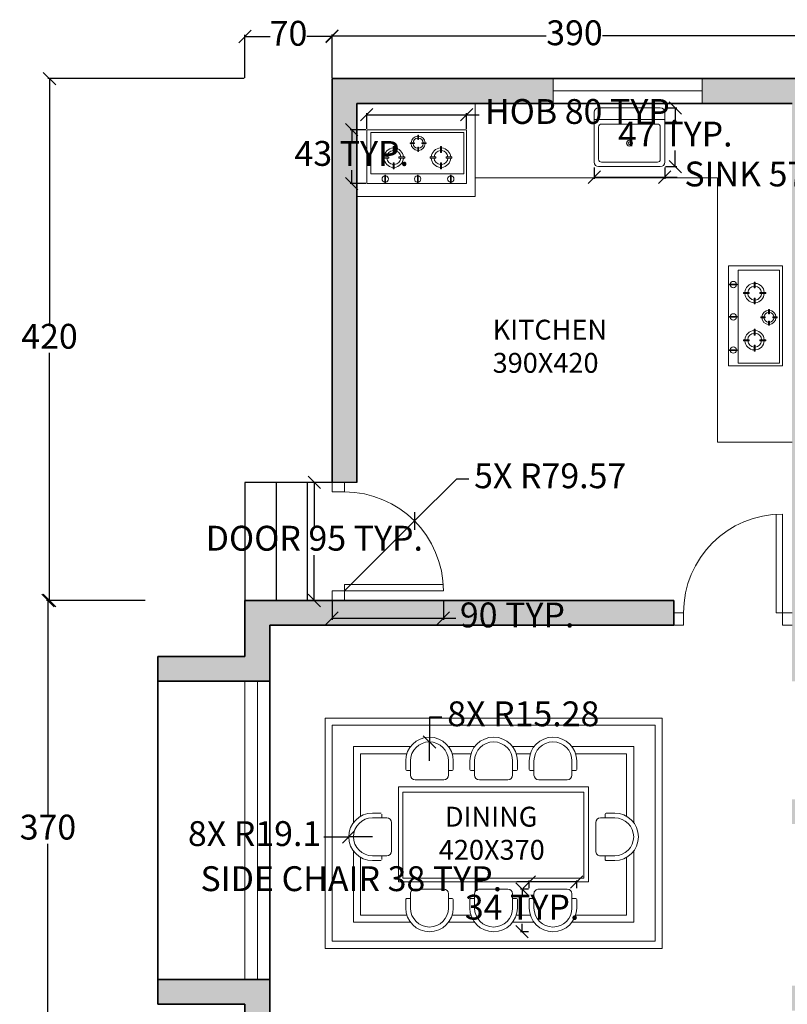
# Model space of a CAD drawing. Units: centimetres. Extents: x 2069 to 3209, y 376 to 1989.
# Tile 2 of 3: x 2069 to 2687, y 1196 to 1989. Entities that reach past the tile are written whole.
import ezdxf

# ---------------------------------------------------------------- set-up
doc = ezdxf.new("R2010")
doc.units = ezdxf.units.CM
for name, color, linetype, lineweight in [('A-ANNO-DIMS', 2, 'Continuous', 18), ('A-AREA-IDEN', 7, 'Continuous', 25), ('A-DOOR', 3, 'Continuous', 18), ('A-EQPM', 8, 'Continuous', 18), ('A-FLOR-CASE', 8, 'Continuous', 18), ('A-FLOR-FIXT', 8, 'Continuous', 18), ('A-FLOR-STRS', 7, 'Continuous', 25), ('A-FURN', 8, 'Continuous', 18), ('A-GLAZ', 4, 'Continuous', 18), ('A-WALL', 7, 'Continuous', 35), ('A-WALL-PATT', 252, 'Continuous', 13)]:
    doc.layers.add(name, color=color, linetype=linetype, lineweight=lineweight)
doc.styles.add('ATTR', font='romans.shx', dxfattribs={"width": 0.8, "height": 1.075})
doc.styles.get("Standard").update_dxf_attribs({"font": 'arial.ttf'})
doc.dimstyles.new('ISO-25', dxfattribs={"dimtxt": 20, "dimasz": 10, "dimexe": 1.25, "dimexo": 0.625, "dimtad": 0, "dimtih": 1, "dimtoh": 1, "dimtxsty": 'Standard', "dimblk": 'OBLIQUE', "dimcen": 6, "dimadec": 0, "dimazin": 0, "dimtfac": 1, "dimtmove": 0, "dimatfit": 3, "dimldrblk": 'OBLIQUE', "dimfxl": 1, "dimarcsym": 0})

# ---------------------------------------------------------------- blocks, each defined once
blk = doc.blocks.new("24'' Sink Single PV")
blk.add_line((-12.00001, -3.999996), (12, -3.999996))
for points in [[(-10.5, 0), (10.5, 0)], [(-12.00001, -18.499996), (-12.00001, -1.5)], [(12, -1.5), (12, -18.499996)], [(-10.5, -17.499996), (-10.5, -6.499996)], [(-9.5, -5.499996), (9.5, -5.499996)], [(10.5, -6.499996), (10.5, -17.499996)], [(10.5, -19.999996), (-10.5, -19.999996)], [(9.5, -18.499996), (-9.5, -18.499996)]]:
    blk.add_lwpolyline(points)
for radius in [1, 0.5]:
    blk.add_circle((0, -11.999996), radius)
for centre, radius, start, end in [((-10.5, -1.5), 1.5, 90, 180), ((10.5, -1.5), 1.5, 0, 90), ((-9.5, -6.499996), 1, 90, 180), ((9.5, -6.499996), 1, 0, 90), ((-10.5, -18.499996), 1.5, 180, 270), ((-9.5, -17.499996), 1, 180, 270), ((9.5, -17.499996), 1, 270, 0), ((10.5, -18.499996), 1.5, 270, 0)]:
    blk.add_arc(centre, radius, start, end)
at = {"style": 'ATTR', "width": 0.8, "flags": 9}
blk.add_attdef('ESTCODE', (0, 0), '', height=0.0048, dxfattribs=at)
blk = doc.blocks.new('A$C72243D80')
at = {"ltscale": 1000}
for p, q in [((0, 0), (0, 384.2)), ((0, 384.2), (712, 384.2)), ((29.5, 68.9), (29.5, 363.2)), ((29.5, 363.2), (692.7, 363.2)), ((692.7, 363.2), (692.7, 68.9)), ((712, 384.2), (712, 0)), ((309.4, 291), (340, 291)), ((309.4, 285), (309.4, 291)), ((340, 285), (309.4, 285)), ((340, 291), (340, 285)), ((363.5, 314.5), (363.5, 345.1)), ((363.5, 345.1), (369.5, 345.1)), ((369.5, 314.5), (363.5, 314.5)), ((369.5, 345.1), (369.5, 314.5)), ((392.3, 291), (392.3, 285)), ((422.9, 291), (392.3, 291)), ((392.3, 285), (422.9, 285)), ((422.9, 285), (422.9, 291)), ((188.1, 264.2), (188.1, 222.1)), ((196.4, 264.2), (188.1, 264.2)), ((188.1, 222.1), (196.4, 222.1)), ((196.4, 222.1), (196.4, 264.2)), ((363.5, 260), (363.5, 229.4)), ((369.5, 260), (363.5, 260)), ((363.5, 229.4), (369.5, 229.4)), ((369.5, 229.4), (369.5, 260)), ((525.9, 222.1), (525.9, 264.2)), ((525.9, 264.2), (534.1, 264.2)), ((534.1, 222.1), (525.9, 222.1)), ((534.1, 264.2), (534.1, 222.1)), ((114.7, 189.8), (156.8, 189.8)), ((114.7, 181.6), (114.7, 189.8)), ((156.8, 181.6), (114.7, 181.6)), ((156.8, 189.8), (156.8, 181.6)), ((188.1, 147.2), (196.4, 147.2)), ((188.1, 105.1), (188.1, 147.2)), ((196.4, 147.2), (196.4, 105.1)), ((228.6, 189.8), (228.6, 181.6)), ((270.7, 189.8), (228.6, 189.8)), ((228.6, 181.6), (270.7, 181.6)), ((270.7, 181.6), (270.7, 189.8)), ((451.5, 189.8), (493.6, 189.8)), ((451.5, 181.6), (451.5, 189.8)), ((493.6, 181.6), (451.5, 181.6)), ((493.6, 189.8), (493.6, 181.6)), ((525.9, 147.2), (525.9, 105.1)), ((534.1, 147.2), (525.9, 147.2)), ((534.1, 105.1), (534.1, 147.2)), ((565.5, 189.8), (565.5, 181.6)), ((607.6, 189.8), (565.5, 189.8)), ((565.5, 181.6), (607.6, 181.6)), ((607.6, 181.6), (607.6, 189.8)), ((196.4, 105.1), (188.1, 105.1)), ((525.9, 105.1), (534.1, 105.1)), ((712, 0), (0, 0)), ((692.7, 68.9), (29.5, 68.9)), ((129.6, 61.1), (129.6, 5)), ((134.4, 61.1), (129.6, 61.1)), ((129.6, 5), (134.4, 5)), ((134.4, 5), (134.4, 61.1)), ((360.9, 5), (360.9, 61.1)), ((360.9, 61.1), (365.7, 61.1)), ((365.7, 5), (360.9, 5)), ((365.7, 61.1), (365.7, 5)), ((597, 5), (597, 61.1)), ((597, 61.1), (601.8, 61.1)), ((601.8, 5), (597, 5)), ((601.8, 61.1), (601.8, 5))]:
    blk.add_line(p, q, dxfattribs=at)
for centre, radius, start, end in [((366.2, 287.2), 50.3, 182.57829, 266.96555), ((366.2, 287.2), 50.3, 93.03445, 175.72709), ((366.1, 287.8), 36.3, 94.03738, 175.01421), ((366.1, 287.8), 36.3, 184.51534, 265.96262), ((366.2, 287.2), 50.3, 4.27291, 86.18384), ((366.1, 287.8), 36.3, 4.98579, 84.5356), ((366.1, 287.8), 36.3, 275.4644, 355.48466), ((366.2, 287.2), 50.3, 273.81616, 357.42171), ((192.7, 184.7), 69.2, 93.81616, 175.72709), ((192.9, 185.5), 49.9, 95.4644, 175.01421), ((192.7, 184.7), 69.2, 4.27291, 86.96555), ((192.9, 185.5), 49.9, 4.98579, 85.96262), ((529.5, 184.7), 69.2, 93.03445, 175.72709), ((529.4, 185.5), 49.9, 94.03738, 175.01421), ((529.5, 184.7), 69.2, 4.27291, 86.18384), ((529.4, 185.5), 49.9, 4.98579, 84.5356), ((192.7, 184.7), 69.2, 182.57829, 266.18384), ((192.9, 185.5), 49.9, 184.51534, 264.5356), ((192.9, 185.5), 49.9, 274.03738, 355.48466), ((192.7, 184.7), 69.2, 273.03445, 357.42171), ((529.5, 184.7), 69.2, 182.57829, 266.96555), ((529.4, 185.5), 49.9, 184.51534, 265.96262), ((529.5, 184.7), 69.2, 273.81616, 357.42171), ((529.4, 185.5), 49.9, 275.4644, 355.48466), ((132.3, 33.2), 22.5, 96.74526, 263.25474), ((132.3, 33.2), 22.5, 275.47893, 84.52107), ((363.1, 33.2), 22.5, 95.47893, 264.52107), ((363.1, 33.2), 22.5, 276.74526, 83.25474), ((599.2, 33.2), 22.5, 95.47893, 264.52107), ((599.2, 33.2), 22.5, 276.74526, 83.25474)]:
    blk.add_arc(centre, radius, start, end, dxfattribs=at)
blk = doc.blocks.new('_Oblique')
at = {"color": 0, "linetype": 'ByBlock', "lineweight": -2}
blk.add_line((-0.5, -0.5), (0.5, 0.5), dxfattribs=at)
blk = doc.blocks.new('*D11')
at = {"layer": 'A-ANNO-DIMS', "color": 0, "lineweight": -2, "transparency": 16777216}
for p, q in [((2320.39, 1941.81), (2320.39, 1976.68)), ((2320.39, 1975.43), (2492.71, 1975.43)), ((2710.39, 1975.43), (2538.06, 1975.43)), ((2710.39, 1941.81), (2710.39, 1976.68))]:
    blk.add_line(p, q, dxfattribs=at)
at = {"layer": 'Defpoints', "color": 0, "transparency": 16777216}
for p in [(2710.39, 1975.43), (2320.39, 1941.18), (2710.39, 1941.18)]:
    blk.add_point(p, dxfattribs=at)
at = {"layer": 'A-ANNO-DIMS', "color": 0, "lineweight": -2, "transparency": 16777216, "xscale": 10, "yscale": 10, "zscale": 10, "rotation": 180}
blk.add_blockref('_Oblique', (2320.39, 1975.43), dxfattribs=at)
at = {"layer": 'A-ANNO-DIMS', "color": 0, "lineweight": -2, "transparency": 16777216, "xscale": 10, "yscale": 10, "zscale": 10}
blk.add_blockref('_Oblique', (2710.39, 1975.43), dxfattribs=at)
at = {"layer": 'A-ANNO-DIMS', "color": 0, "transparency": 16777216, "insert": (2515.39, 1975.43), "char_height": 20, "attachment_point": 5}
blk.add_mtext('390', dxfattribs=at)
blk = doc.blocks.new('*D14')
at = {"layer": 'A-ANNO-DIMS', "color": 0, "lineweight": -2, "transparency": 16777216}
for p, q in [((2250.39, 1941.81), (2250.39, 1976.27)), ((2250.39, 1975.02), (2270.55, 1975.02)), ((2320.39, 1975.02), (2300.22, 1975.02)), ((2320.39, 1941.81), (2320.39, 1976.27))]:
    blk.add_line(p, q, dxfattribs=at)
at = {"layer": 'Defpoints', "color": 0, "transparency": 16777216}
for p in [(2320.39, 1975.02), (2250.39, 1941.18), (2320.39, 1941.18)]:
    blk.add_point(p, dxfattribs=at)
at = {"layer": 'A-ANNO-DIMS', "color": 0, "lineweight": -2, "transparency": 16777216, "xscale": 10, "yscale": 10, "zscale": 10, "rotation": 180}
blk.add_blockref('_Oblique', (2250.39, 1975.02), dxfattribs=at)
at = {"layer": 'A-ANNO-DIMS', "color": 0, "lineweight": -2, "transparency": 16777216, "xscale": 10, "yscale": 10, "zscale": 10}
blk.add_blockref('_Oblique', (2320.39, 1975.02), dxfattribs=at)
at = {"layer": 'A-ANNO-DIMS', "color": 0, "transparency": 16777216, "insert": (2285.39, 1975.02), "char_height": 20, "attachment_point": 5}
blk.add_mtext('70', dxfattribs=at)
blk = doc.blocks.new('*D20')
at = {"layer": 'A-ANNO-DIMS', "color": 0, "lineweight": -2, "transparency": 16777216}
for p, q in [((2249.76, 1941.18), (2091.91, 1941.18)), ((2093.16, 1941.18), (2093.16, 1742.02)), ((2093.16, 1521.18), (2093.16, 1720.35)), ((2170.21, 1521.18), (2091.91, 1521.18))]:
    blk.add_line(p, q, dxfattribs=at)
at = {"layer": 'Defpoints', "color": 0, "transparency": 16777216}
for p in [(2250.39, 1941.18), (2093.16, 1521.18), (2170.84, 1521.18)]:
    blk.add_point(p, dxfattribs=at)
at = {"layer": 'A-ANNO-DIMS', "color": 0, "lineweight": -2, "transparency": 16777216, "xscale": 10, "yscale": 10, "zscale": 10}
for p, rotation in [((2093.16, 1941.18), 90), ((2093.16, 1521.18), 270)]:
    blk.add_blockref('_Oblique', p, dxfattribs=dict(at, rotation=rotation))
at = {"layer": 'A-ANNO-DIMS', "color": 0, "transparency": 16777216, "insert": (2093.16, 1731.18), "char_height": 20, "attachment_point": 5}
blk.add_mtext('420', dxfattribs=at)
blk = doc.blocks.new('*D21')
at = {"layer": 'A-ANNO-DIMS', "color": 0, "lineweight": -2, "transparency": 16777216}
for p, q in [((2170.21, 1521.18), (2090.66, 1521.18)), ((2091.91, 1521.18), (2091.91, 1347.03)), ((2091.91, 1151.18), (2091.91, 1325.34)), ((2171.09, 1151.18), (2090.66, 1151.18))]:
    blk.add_line(p, q, dxfattribs=at)
at = {"layer": 'Defpoints', "color": 0, "transparency": 16777216}
for p in [(2170.84, 1521.18), (2091.91, 1151.18), (2171.71, 1151.18)]:
    blk.add_point(p, dxfattribs=at)
at = {"layer": 'A-ANNO-DIMS', "color": 0, "lineweight": -2, "transparency": 16777216, "xscale": 10, "yscale": 10, "zscale": 10}
for p, rotation in [((2091.91, 1521.18), 90), ((2091.91, 1151.18), 270)]:
    blk.add_blockref('_Oblique', p, dxfattribs=dict(at, rotation=rotation))
at = {"layer": 'A-ANNO-DIMS', "color": 0, "transparency": 16777216, "insert": (2091.91, 1336.18), "char_height": 20, "attachment_point": 5}
blk.add_mtext('370', dxfattribs=at)
blk = doc.blocks.new('CHAIR-DINING')
for p, q in [((0, 8.4), (0, 15.28)), ((3.82, 15.28), (3.82, 3.82)), ((34.38, 3.82), (34.38, 15.28)), ((38.2, 8.4), (38.2, 15.28)), ((0.76, 7.64), (3.82, 7.64)), ((34.38, 7.64), (37.43, 7.64)), ((7.64, 0), (30.56, 0))]:
    blk.add_line(p, q)
for centre, radius, start, end in [((19.1, 15.28), 19.1, 0, 180), ((19.1, 15.28), 15.28, 0.00007, 179.99993), ((0.76, 8.4), 0.764, 180, 270), ((37.43, 8.4), 0.764, 270, 0), ((7.64, 3.82), 3.82, 180, 270), ((30.56, 3.82), 3.82, 270, 0)]:
    blk.add_arc(centre, radius, start, end)
blk = doc.blocks.new('DOOR-SINGLE-950')
for p, q in [((82.28, 89.41), (82.28, 10)), ((87.28, 89.57), (87.28, 10)), ((0, 10), (7.71, 10)), ((7.71, 10), (7.71, 0)), ((82.28, 10), (87.28, 10)), ((95, 10), (87.28, 10)), ((87.28, 10), (87.28, 0)), ((7.71, 0), (0, 0)), ((87.28, 0), (95, 0))]:
    blk.add_line(p, q)
blk.add_arc((87.28, 10), 79.57, 90, 180)
blk = doc.blocks.new('*D28')
at = {"layer": 'A-ANNO-DIMS', "color": 0, "lineweight": -2, "transparency": 16777216}
for p, q in [((2478.99, 1294.68), (2468.99, 1294.68)), ((2478.99, 1289.57), (2478.99, 1295.93)), ((2517.18, 1294.68), (2478.99, 1294.68)), ((2517.18, 1289.57), (2517.18, 1295.93))]:
    blk.add_line(p, q, dxfattribs=at)
at = {"layer": 'Defpoints', "color": 0, "transparency": 16777216}
for p in [(2478.99, 1294.68), (2478.99, 1288.95), (2517.18, 1288.95)]:
    blk.add_point(p, dxfattribs=at)
at = {"layer": 'A-ANNO-DIMS', "color": 0, "lineweight": -2, "transparency": 16777216, "xscale": 10, "yscale": 10, "zscale": 10, "rotation": 180}
blk.add_blockref('_Oblique', (2478.99, 1294.68), dxfattribs=at)
at = {"layer": 'A-ANNO-DIMS', "color": 0, "lineweight": -2, "transparency": 16777216, "xscale": 10, "yscale": 10, "zscale": 10}
blk.add_blockref('_Oblique', (2517.18, 1294.68), dxfattribs=at)
at = {"layer": 'A-ANNO-DIMS', "color": 0, "transparency": 16777216, "insert": (2335.9, 1294.68), "char_height": 20, "attachment_point": 5}
blk.add_mtext('SIDE CHAIR 38 TYP.', dxfattribs=at)
blk = doc.blocks.new('*D29')
at = {"layer": 'A-ANNO-DIMS', "color": 0, "lineweight": -2, "transparency": 16777216}
for p, q in [((2478.36, 1288.95), (2472.01, 1288.95)), ((2473.26, 1288.95), (2473.26, 1282.6)), ((2473.26, 1254.57), (2473.26, 1260.91)), ((2478.36, 1254.57), (2472.01, 1254.57))]:
    blk.add_line(p, q, dxfattribs=at)
at = {"layer": 'Defpoints', "color": 0, "transparency": 16777216}
for p in [(2478.99, 1288.95), (2473.26, 1254.57), (2478.99, 1254.57)]:
    blk.add_point(p, dxfattribs=at)
at = {"layer": 'A-ANNO-DIMS', "color": 0, "lineweight": -2, "transparency": 16777216, "xscale": 10, "yscale": 10, "zscale": 10}
for p, rotation in [((2473.26, 1288.95), 90), ((2473.26, 1254.57), 270)]:
    blk.add_blockref('_Oblique', p, dxfattribs=dict(at, rotation=rotation))
at = {"layer": 'A-ANNO-DIMS', "color": 0, "transparency": 16777216, "insert": (2473.26, 1271.76), "char_height": 20, "attachment_point": 5}
blk.add_mtext('34 TYP.', dxfattribs=at)
blk = doc.blocks.new('*D30')
at = {"layer": 'A-ANNO-DIMS', "color": 0, "lineweight": -2, "transparency": 16777216}
for p, q in [((2319.76, 1616.18), (2304.89, 1616.18)), ((2306.14, 1616.18), (2306.14, 1579.65)), ((2306.14, 1521.18), (2306.14, 1557.71)), ((2319.76, 1521.18), (2304.89, 1521.18))]:
    blk.add_line(p, q, dxfattribs=at)
at = {"layer": 'Defpoints', "color": 0, "transparency": 16777216}
for p in [(2320.39, 1616.18), (2306.14, 1521.18), (2320.39, 1521.18)]:
    blk.add_point(p, dxfattribs=at)
at = {"layer": 'A-ANNO-DIMS', "color": 0, "lineweight": -2, "transparency": 16777216, "xscale": 10, "yscale": 10, "zscale": 10}
for p, rotation in [((2306.14, 1616.18), 90), ((2306.14, 1521.18), 270)]:
    blk.add_blockref('_Oblique', p, dxfattribs=dict(at, rotation=rotation))
at = {"layer": 'A-ANNO-DIMS', "color": 0, "transparency": 16777216, "insert": (2306.14, 1568.68), "char_height": 20, "attachment_point": 5}
blk.add_mtext('DOOR 95 TYP.', dxfattribs=at)
blk = doc.blocks.new('*D31')
at = {"layer": 'A-ANNO-DIMS', "color": 0, "lineweight": -2, "transparency": 16777216}
for p, q in [((2320.39, 1520.56), (2320.39, 1505.68)), ((2409.96, 1520.56), (2409.96, 1505.68)), ((2320.39, 1506.93), (2409.96, 1506.93)), ((2409.96, 1506.93), (2419.96, 1506.93))]:
    blk.add_line(p, q, dxfattribs=at)
at = {"layer": 'Defpoints', "color": 0, "transparency": 16777216}
for p in [(2320.39, 1521.18), (2409.96, 1521.18), (2409.96, 1506.93)]:
    blk.add_point(p, dxfattribs=at)
at = {"layer": 'A-ANNO-DIMS', "color": 0, "lineweight": -2, "transparency": 16777216, "xscale": 10, "yscale": 10, "zscale": 10, "rotation": 180}
blk.add_blockref('_Oblique', (2320.39, 1506.93), dxfattribs=at)
at = {"layer": 'A-ANNO-DIMS', "color": 0, "lineweight": -2, "transparency": 16777216, "xscale": 10, "yscale": 10, "zscale": 10}
blk.add_blockref('_Oblique', (2409.96, 1506.93), dxfattribs=at)
at = {"layer": 'A-ANNO-DIMS', "color": 0, "transparency": 16777216, "insert": (2469.26, 1506.93), "char_height": 20, "attachment_point": 5}
blk.add_mtext('90 TYP.', dxfattribs=at)
blk = doc.blocks.new('*D36')
at = {"layer": 'A-ANNO-DIMS', "color": 0, "lineweight": -2, "transparency": 16777216}
for p, q in [((2531.27, 1869.68), (2531.27, 1860.55)), ((2587.96, 1869.68), (2587.96, 1860.55)), ((2531.27, 1861.8), (2587.96, 1861.8)), ((2587.96, 1861.8), (2597.96, 1861.8))]:
    blk.add_line(p, q, dxfattribs=at)
at = {"layer": 'Defpoints', "color": 0, "transparency": 16777216}
for p in [(2531.27, 1870.31), (2587.96, 1870.31), (2587.96, 1861.8)]:
    blk.add_point(p, dxfattribs=at)
at = {"layer": 'A-ANNO-DIMS', "color": 0, "lineweight": -2, "transparency": 16777216, "xscale": 10, "yscale": 10, "zscale": 10, "rotation": 180}
blk.add_blockref('_Oblique', (2531.27, 1861.8), dxfattribs=at)
at = {"layer": 'A-ANNO-DIMS', "color": 0, "lineweight": -2, "transparency": 16777216, "xscale": 10, "yscale": 10, "zscale": 10}
blk.add_blockref('_Oblique', (2587.96, 1861.8), dxfattribs=at)
at = {"layer": 'A-ANNO-DIMS', "color": 0, "transparency": 16777216, "insert": (2683.7, 1861.8), "char_height": 20, "attachment_point": 5}
blk.add_mtext('SINK 57 TYP.', dxfattribs=at)
blk = doc.blocks.new('*D37')
at = {"layer": 'A-ANNO-DIMS', "color": 0, "lineweight": -2, "transparency": 16777216}
for p, q in [((2588.59, 1917.56), (2597.72, 1917.56)), ((2596.47, 1917.56), (2596.47, 1904.57)), ((2596.47, 1870.31), (2596.47, 1883.3)), ((2588.59, 1870.31), (2597.72, 1870.31))]:
    blk.add_line(p, q, dxfattribs=at)
at = {"layer": 'Defpoints', "color": 0, "transparency": 16777216}
for p in [(2587.96, 1917.56), (2596.47, 1917.56), (2587.96, 1870.31)]:
    blk.add_point(p, dxfattribs=at)
at = {"layer": 'A-ANNO-DIMS', "color": 0, "lineweight": -2, "transparency": 16777216, "xscale": 10, "yscale": 10, "zscale": 10}
for p, rotation in [((2596.47, 1917.56), 90), ((2596.47, 1870.31), 270)]:
    blk.add_blockref('_Oblique', p, dxfattribs=dict(at, rotation=rotation))
at = {"layer": 'A-ANNO-DIMS', "color": 0, "transparency": 16777216, "insert": (2596.47, 1893.93), "char_height": 20, "attachment_point": 5}
blk.add_mtext('47 TYP.', dxfattribs=at)
blk = doc.blocks.new('*D38')
at = {"layer": 'A-ANNO-DIMS', "color": 0, "lineweight": -2, "transparency": 16777216}
for p, q in [((2348.29, 1900.65), (2348.29, 1913.33)), ((2348.29, 1912.08), (2428.64, 1912.08)), ((2428.64, 1900.65), (2428.64, 1913.33)), ((2428.64, 1912.08), (2438.64, 1912.08))]:
    blk.add_line(p, q, dxfattribs=at)
at = {"layer": 'Defpoints', "color": 0, "transparency": 16777216}
for p in [(2428.64, 1912.08), (2348.29, 1900.03), (2428.64, 1900.03)]:
    blk.add_point(p, dxfattribs=at)
at = {"layer": 'A-ANNO-DIMS', "color": 0, "lineweight": -2, "transparency": 16777216, "xscale": 10, "yscale": 10, "zscale": 10, "rotation": 180}
blk.add_blockref('_Oblique', (2348.29, 1912.08), dxfattribs=at)
at = {"layer": 'A-ANNO-DIMS', "color": 0, "lineweight": -2, "transparency": 16777216, "xscale": 10, "yscale": 10, "zscale": 10}
blk.add_blockref('_Oblique', (2428.64, 1912.08), dxfattribs=at)
at = {"layer": 'A-ANNO-DIMS', "color": 0, "transparency": 16777216, "insert": (2521.55, 1912.08), "char_height": 20, "attachment_point": 5}
blk.add_mtext('HOB 80 TYP.', dxfattribs=at)
blk = doc.blocks.new('*D39')
at = {"layer": 'A-ANNO-DIMS', "color": 0, "lineweight": -2, "transparency": 16777216}
for p, q in [((2347.66, 1900.03), (2334.98, 1900.03)), ((2336.23, 1900.03), (2336.23, 1889.19)), ((2336.23, 1856.67), (2336.23, 1867.51)), ((2347.66, 1856.67), (2334.98, 1856.67))]:
    blk.add_line(p, q, dxfattribs=at)
at = {"layer": 'Defpoints', "color": 0, "transparency": 16777216}
for p in [(2336.23, 1900.03), (2348.29, 1900.03), (2348.29, 1856.67)]:
    blk.add_point(p, dxfattribs=at)
at = {"layer": 'A-ANNO-DIMS', "color": 0, "lineweight": -2, "transparency": 16777216, "xscale": 10, "yscale": 10, "zscale": 10}
for p, rotation in [((2336.23, 1900.03), 90), ((2336.23, 1856.67), 270)]:
    blk.add_blockref('_Oblique', p, dxfattribs=dict(at, rotation=rotation))
at = {"layer": 'A-ANNO-DIMS', "color": 0, "transparency": 16777216, "insert": (2336.23, 1878.35), "char_height": 20, "attachment_point": 5}
blk.add_mtext('43 TYP.', dxfattribs=at)
blk = doc.blocks.new('*D50')
at = {"layer": 'A-ANNO-DIMS', "color": 0, "lineweight": -2, "transparency": 16777216}
for p, q in [((2420.41, 1618.92), (2386.65, 1585.16)), ((2430.41, 1618.92), (2420.41, 1618.92)), ((2330.39, 1528.9), (2386.65, 1585.16))]:
    blk.add_line(p, q, dxfattribs=at)
at = {"layer": 'Defpoints', "color": 0, "transparency": 16777216}
for p in [(2386.65, 1585.16), (2330.39, 1528.9)]:
    blk.add_point(p, dxfattribs=at)
at = {"layer": 'A-ANNO-DIMS', "color": 0, "lineweight": -2, "transparency": 16777216, "xscale": 10, "yscale": 10, "zscale": 10, "rotation": 224.9997739305666}
blk.add_blockref('_Oblique', (2386.65, 1585.16), dxfattribs=at)
at = {"layer": 'A-ANNO-DIMS', "color": 0, "transparency": 16777216, "insert": (2495.84, 1618.92), "char_height": 20, "attachment_point": 5}
blk.add_mtext('5X R79.57', dxfattribs=at)
blk = doc.blocks.new('*D55')
at = {"layer": 'A-ANNO-DIMS', "color": 0, "lineweight": -2, "transparency": 16777216}
for p in [(2313.84, 1330.96), (2352.94, 1330.96)]:
    blk.add_line(p, (2333.84, 1330.96), dxfattribs=at)
at = {"layer": 'Defpoints', "color": 0, "transparency": 16777216}
for p in [(2333.84, 1330.96), (2352.94, 1330.96)]:
    blk.add_point(p, dxfattribs=at)
at = {"layer": 'A-ANNO-DIMS', "color": 0, "lineweight": -2, "transparency": 16777216, "xscale": 10, "yscale": 10, "zscale": 10, "rotation": 359.9994809913539}
blk.add_blockref('_Oblique', (2333.84, 1330.96), dxfattribs=at)
at = {"layer": 'A-ANNO-DIMS', "color": 0, "transparency": 16777216, "insert": (2258.1, 1330.96), "char_height": 20, "attachment_point": 5}
blk.add_mtext('8X R19.1', dxfattribs=at)
blk = doc.blocks.new('*D56')
at = {"layer": 'A-ANNO-DIMS', "color": 0, "lineweight": -2, "transparency": 16777216}
for p, q in [((2408.77, 1427.36), (2398.77, 1427.36)), ((2398.77, 1427.36), (2398.77, 1407.36)), ((2398.77, 1392.08), (2398.77, 1407.36))]:
    blk.add_line(p, q, dxfattribs=at)
at = {"layer": 'Defpoints', "color": 0, "transparency": 16777216}
for p in [(2398.77, 1407.36), (2398.77, 1392.08)]:
    blk.add_point(p, dxfattribs=at)
at = {"layer": 'A-ANNO-DIMS', "color": 0, "lineweight": -2, "transparency": 16777216, "xscale": 10, "yscale": 10, "zscale": 10, "rotation": 269.9993737395664}
blk.add_blockref('_Oblique', (2398.77, 1407.36), dxfattribs=at)
at = {"layer": 'A-ANNO-DIMS', "color": 0, "transparency": 16777216, "insert": (2474.23, 1427.36), "char_height": 20, "attachment_point": 5}
blk.add_mtext('8X R15.28', dxfattribs=at)

msp = doc.modelspace()

# ---------------------------------------------------------------- hatches: boundary and pattern name
at = {"layer": 'A-WALL-PATT'}
h = msp.add_hatch(color=256, dxfattribs=at)
h.dxf.hatch_style = 1
h.paths.add_polyline_path([(2498.1872, 1921.1819), (2498.1872, 1941.1819), (2320.3865, 1941.1819), (2320.3865, 1616.1819), (2340.3865, 1616.1819), (2340.3865, 1921.1819)])
h.paths.add_polyline_path([(2690.3865, 1921.1819), (2690.3865, 1456.1819), (2710.3865, 1456.1819), (2710.3865, 1741.1819), (2742.2674, 1741.1819), (2742.2674, 1761.1819), (2710.3865, 1761.1819), (2710.3865, 1941.1819), (2618.1872, 1941.1819), (2618.1872, 1921.1819)])
h.paths.add_polyline_path([(2802.2674, 1761.1819), (2802.2674, 1741.1819), (2971.3879, 1741.1819), (2971.3879, 1761.1819)])
h.paths.add_polyline_path([(3080.3865, 1761.1819), (3031.3879, 1761.1819), (3031.3879, 1741.1819), (3060.3865, 1741.1819), (3060.3865, 1621.1819), (3080.3865, 1621.1819)])
h.paths.add_polyline_path([(3060.3865, 1361.1819), (2906.9077, 1361.1819), (2906.9077, 1341.1819), (3060.3865, 1341.1819), (3060.3865, 1296.1819), (3080.3865, 1296.1819), (3080.3865, 1481.1819), (3060.3865, 1481.1819)])
h.paths.add_polyline_path([(2799.9077, 1341.1819), (2799.9077, 1211.1819), (2690.3865, 1211.1819), (2690.3865, 1191.1819), (3060.3865, 1191.1819), (3060.3865, 1131.1819), (3080.3865, 1131.1819), (3080.3865, 1256.1819), (3060.3865, 1256.1819), (3060.3865, 1211.1819), (2821.9077, 1211.1819), (2821.9077, 1361.1819), (2690.3865, 1361.1819), (2690.3865, 1341.1819)])
h.paths.add_polyline_path([(3080.3865, 1051.1819), (3060.3865, 1051.1819), (3060.3865, 991.1819), (2805.3865, 991.1819), (2805.3865, 971.1819), (3060.3865, 971.1819), (3060.3865, 861.1819), (3080.3865, 861.1819)])
h.paths.add_polyline_path([(2690.3865, 591.1819), (2815.3865, 591.1819), (2815.3865, 611.1819), (2710.3865, 611.1819), (2710.3865, 991.1819), (2690.3865, 991.1819)])
h.paths.add_polyline_path([(2955.3865, 611.1819), (2955.3865, 591.1819), (3080.3865, 591.1819), (3080.3865, 721.1819), (3060.3865, 721.1819), (3060.3865, 611.1819)])
h.paths.add_polyline_path([(2320.3865, 656.2562), (2320.3865, 639.1819), (2343.1963, 639.1819), (2343.1963, 656.2562)])
h.paths.add_polyline_path([(2320.3865, 863.2574), (2250.3865, 863.2574), (2250.3865, 841.2574), (2407.8865, 841.2574), (2407.8865, 863.2574), (2340.3865, 863.2574), (2340.3865, 927.2197), (2320.3865, 927.2197)])
h.paths.add_polyline_path([(2320.3865, 1151.1819), (2320.3865, 1087.2197), (2340.3865, 1087.2197), (2340.3865, 1151.1819), (2595.3865, 1151.1819), (2595.3865, 1171.1819), (2270.3865, 1171.1819), (2270.3865, 1216.1819), (2180.3865, 1216.1819), (2180.3865, 1196.1819), (2250.3865, 1196.1819), (2250.3865, 1151.1819)])
h.paths.add_polyline_path([(2595.3865, 1501.1819), (2595.3865, 1521.1819), (2250.3865, 1521.1819), (2250.3865, 1476.1819), (2180.3865, 1476.1819), (2180.3865, 1456.1819), (2270.3865, 1456.1819), (2270.3865, 1501.1819)])

# ---------------------------------------------------------------- linework, layer by layer
at = {"layer": 'A-FLOR-CASE'}
for p, q in [((2435.3865, 1921.1819), (2435.3865, 1846.1819)), ((2435.3865, 1861.1819), (2630.3865, 1861.1819)), ((2630.3865, 1861.1819), (2630.3865, 1648.6184)), ((2340.3865, 1846.1819), (2435.3865, 1846.1819)), ((2630.3865, 1648.6184), (2690.3865, 1648.6184))]:
    msp.add_line(p, q, dxfattribs=at)
at = {"layer": 'A-FLOR-STRS'}
for p, q in [((2340.3865, 1616.1819), (2250.3865, 1616.1819)), ((2250.3865, 1616.1819), (2250.3865, 1521.1819)), ((2275.3865, 1616.1819), (2275.3865, 1521.1819)), ((2300.3865, 1616.1819), (2300.3865, 1521.1819))]:
    msp.add_line(p, q, dxfattribs=at)
at = {"layer": 'A-FURN'}
for p, q in [((2585.9359, 1426.4542), (2314.7404, 1426.4542)), ((2314.7404, 1426.4542), (2314.7404, 1241.2009)), ((2585.9359, 1241.2009), (2585.9359, 1426.4542)), ((2580.2064, 1420.7247), (2320.4699, 1420.7247)), ((2320.4699, 1420.7247), (2320.4699, 1246.9304)), ((2580.2064, 1246.9304), (2580.2064, 1420.7247)), ((2383.4942, 1403.5363), (2337.6584, 1403.5363)), ((2337.6584, 1403.5363), (2337.6584, 1342.4218)), ((2435.0596, 1403.5363), (2414.0515, 1403.5363)), ((2482.8052, 1403.5363), (2465.6168, 1403.5363)), ((2563.018, 1403.5363), (2513.3625, 1403.5363)), ((2563.018, 1342.4218), (2563.018, 1403.5363)), ((2343.3878, 1397.8068), (2343.3878, 1347.5024)), ((2380.5542, 1397.8068), (2343.3878, 1397.8068)), ((2432.1196, 1397.8068), (2416.9914, 1397.8068)), ((2479.8653, 1397.8068), (2468.5568, 1397.8068)), ((2557.2885, 1397.8068), (2516.3025, 1397.8068)), ((2557.2885, 1347.5024), (2557.2885, 1397.8068)), ((2373.9451, 1294.6761), (2373.9451, 1371.0692)), ((2373.9451, 1371.0692), (2526.7313, 1371.0692)), ((2526.7313, 1371.0692), (2526.7313, 1294.6761)), ((2359.8124, 1350.0611), (2352.937, 1350.0611)), ((2360.5763, 1346.2414), (2360.5763, 1349.2972)), ((2364.3959, 1346.2414), (2352.937, 1346.2414)), ((2368.2156, 1319.5039), (2368.2156, 1342.4218)), ((2337.6584, 1319.5039), (2337.6584, 1262.209)), ((2352.937, 1315.6842), (2364.3959, 1315.6842)), ((2360.5763, 1312.6285), (2360.5763, 1315.6842)), ((2563.018, 1262.209), (2563.018, 1319.5039)), ((2343.3878, 1314.4232), (2343.3878, 1267.9385)), ((2359.8124, 1311.8646), (2352.937, 1311.8646)), ((2557.2885, 1267.9385), (2557.2885, 1314.4232)), ((2526.7313, 1294.6761), (2373.9451, 1294.6761)), ((2343.3878, 1267.9385), (2380.5542, 1267.9385)), ((2416.9914, 1267.9385), (2432.1196, 1267.9385)), ((2468.5568, 1267.9385), (2479.8653, 1267.9385)), ((2516.3025, 1267.9385), (2557.2885, 1267.9385)), ((2337.6584, 1262.209), (2383.4942, 1262.209)), ((2414.0515, 1262.209), (2435.0596, 1262.209)), ((2465.6168, 1262.209), (2482.8052, 1262.209)), ((2513.3625, 1262.209), (2563.018, 1262.209)), ((2320.4699, 1246.9304), (2580.2064, 1246.9304)), ((2314.7404, 1241.2009), (2585.9359, 1241.2009))]:
    msp.add_line(p, q, dxfattribs=at)
msp.add_lwpolyline([(2377.3409, 1366.9642), (2522.9512, 1366.9642), (2522.9512, 1297.7838), (2377.3409, 1297.7838)], close=True, dxfattribs=at)
for centre, radius, start, end in [((2352.937, 1330.9628), 19.0983, 90, 270), ((2352.937, 1330.9628), 15.2786, 90.0000737, 269.9999263), ((2364.3959, 1342.4218), 3.8197, 0, 90), ((2364.3959, 1319.5039), 3.8197, 270, 0)]:
    msp.add_arc(centre, radius, start, end, dxfattribs=at)
at = {"layer": 'A-GLAZ'}
for p, q in [((2498.1872, 1921.1819), (2498.1872, 1941.1819)), ((2618.1872, 1921.1819), (2618.1872, 1941.1819)), ((2498.1872, 1931.1819), (2618.1872, 1931.1819)), ((2250.3865, 1456.1819), (2250.3865, 1216.1819)), ((2260.3865, 1216.1819), (2260.3865, 1456.1819))]:
    msp.add_line(p, q, dxfattribs=at)
at = {"layer": 'A-WALL'}
for p, q in [((2320.3865, 1941.1819), (2710.3865, 1941.1819)), ((2320.3865, 1941.1819), (2320.3865, 1616.1819)), ((2340.3865, 1921.1819), (2690.3865, 1921.1819)), ((2340.3865, 1921.1819), (2340.3865, 1616.1819)), ((2595.3865, 1521.1819), (2250.3865, 1521.1819)), ((2250.3865, 1521.1819), (2250.3865, 1476.1819)), ((2595.3865, 1521.1819), (2595.3865, 1501.1819)), ((2595.3865, 1501.1819), (2270.3865, 1501.1819)), ((2270.3865, 1501.1819), (2270.3865, 1171.1819)), ((2180.3865, 1476.1819), (2180.3865, 1196.1819)), ((2250.3865, 1476.1819), (2180.3865, 1476.1819)), ((2270.3865, 1456.1819), (2180.3865, 1456.1819)), ((2270.3865, 1216.1819), (2180.3865, 1216.1819)), ((2250.3865, 1196.1819), (2180.3865, 1196.1819)), ((2250.3865, 1196.1819), (2250.3865, 841.2574))]:
    msp.add_line(p, q, dxfattribs=at)

# ---------------------------------------------------------------- block references
at = {"layer": 'A-DOOR', "rotation": 269.9999999999997}
msp.add_blockref('DOOR-SINGLE-950', (2320.3866, 1616.1815), dxfattribs=at)
at = {"layer": 'A-DOOR'}
msp.add_blockref('DOOR-SINGLE-950', (2595.387, 1501.182), dxfattribs=at)
at = {"layer": 'A-EQPM', "xscale": 0.1128460274394379, "yscale": 0.1128460274394379, "zscale": 0.1128460274394379}
msp.add_blockref('A$C72243D80', (2348.2865, 1856.6729), dxfattribs=at)
at = {"layer": 'A-EQPM', "xscale": 0.1128460274394379, "yscale": 0.1128460274394379, "zscale": 0.1128460274394379, "rotation": 270}
msp.add_blockref('A$C72243D80', (2639.3664, 1790.3423), dxfattribs=at)
at = {"layer": 'A-FLOR-FIXT', "xscale": 2.362111345995379, "yscale": 2.362111345995379, "zscale": 2.362111345995379}
msp.add_blockref("24'' Sink Single PV", (2559.6171, 1917.5491), dxfattribs=at)
at = {"layer": 'A-FURN'}
for p in [(2379.675, 1376.799), (2431.2403, 1376.799), (2478.986, 1376.799)]:
    msp.add_blockref('CHAIR-DINING', p, dxfattribs=at)
for p, rotation in [((2532.4611, 1350.0607), 270.000000000189), ((2417.8707, 1288.9463), 180), ((2469.436, 1288.9463), 180), ((2517.1817, 1288.9463), 180)]:
    msp.add_blockref('CHAIR-DINING', p, dxfattribs=dict(at, rotation=rotation))

# ---------------------------------------------------------------- texts
at = {"layer": 'A-AREA-IDEN', "char_height": 16, "attachment_point": 1}
for s, width, insert in [('KITCHEN\\P390X420', 109.524929, (2449.5532, 1747.0716)), (' DINING\\P420X370', 112.813406, (2406.2964, 1355.1715))]:
    msp.add_mtext_dynamic_manual_height_columns(s, width=width, gutter_width=12.5, heights=[0], dxfattribs=dict(at, insert=insert))

# ---------------------------------------------------------------- dimensions: what is measured, and where the dimension line sits
at = {"layer": 'A-ANNO-DIMS'}
for base, p1, p2, picture, middle in [((2320.3865, 1975.0194), (2250.3865, 1941.1819), (2320.3865, 1941.1819), '*D14', (2285.3865, 1975.0194)), ((2710.3865, 1975.4288), (2320.3865, 1941.1819), (2710.3865, 1941.1819), '*D11', (2515.3865, 1975.4288))]:
    dim = msp.add_linear_dim(base=base, p1=p1, p2=p2, dimstyle='ISO-25', override={"dimclrd": 0, "dimclre": 0, "dimclrt": 0}, dxfattribs=at)
    dim.commit()
    dim.dimension.update_dxf_attribs({"geometry": picture, "text_midpoint": middle})
for base, p1, p2, text, picture, middle in [((2428.638, 1912.0817), (2348.2865, 1900.029), (2428.638, 1900.029), 'HOB <> TYP.', '*D38', (2521.555, 1912.0817)), ((2587.9624, 1861.8033), (2531.2717, 1870.3069), (2587.9624, 1870.3069), 'SINK <> TYP.', '*D36', (2683.7034, 1861.8033)), ((2409.9564, 1506.9319), (2320.3865, 1521.1819), (2409.9564, 1521.1819), '<> TYP.', '*D31', (2469.2581, 1506.9319))]:
    dim = msp.add_linear_dim(base=base, p1=p1, p2=p2, text=text, dimstyle='ISO-25', override={"dimdec": 0, "dimlfac": 1, "dimrnd": 0, "dimzin": 0, "dimdsep": 46, "dimlunit": 2}, dxfattribs=at)
    dim.commit()
    dim.dimension.update_dxf_attribs({"geometry": picture, "text_midpoint": middle})
for base, p1, p2, picture, middle in [((2093.1605, 1521.1819), (2250.3865, 1941.1819), (2170.836, 1521.1819), '*D20', (2093.1605, 1731.1819)), ((2091.9105, 1151.1819), (2170.836, 1521.1819), (2171.711, 1151.1819), '*D21', (2091.9105, 1336.1819))]:
    dim = msp.add_linear_dim(base=base, p1=p1, p2=p2, angle=90, dimstyle='ISO-25', override={"dimclrd": 0, "dimclre": 0, "dimclrt": 0}, dxfattribs=at)
    dim.commit()
    dim.dimension.update_dxf_attribs({"geometry": picture, "text_midpoint": middle})
for base, p1, p2, angle, text, picture, middle in [((2596.466, 1917.5605), (2587.9624, 1870.3069), (2587.9624, 1917.5605), 90, '<> TYP.', '*D37', (2596.466, 1893.9337)), ((2336.2337, 1900.029), (2348.2865, 1856.6729), (2348.2865, 1900.029), 90, '<> TYP.', '*D39', (2336.2337, 1878.351)), ((2306.1365, 1521.1819), (2320.3865, 1616.1819), (2320.3865, 1521.1819), 270, 'DOOR <> TYP.', '*D30', (2306.1365, 1568.6819)), ((2478.9856, 1294.6761), (2517.1821, 1288.9466), (2478.9856, 1288.9466), 180, 'SIDE CHAIR <> TYP.', '*D28', (2335.8981, 1294.6761)), ((2473.2561, 1254.5697), (2478.9856, 1288.9466), (2478.9856, 1254.5697), 270, '<> TYP.', '*D29', (2473.2561, 1271.7582))]:
    dim = msp.add_linear_dim(base=base, p1=p1, p2=p2, angle=angle, text=text, dimstyle='ISO-25', override={"dimdec": 0, "dimlfac": 1, "dimrnd": 0, "dimzin": 0, "dimdsep": 46, "dimlunit": 2}, dxfattribs=at)
    dim.commit()
    dim.dimension.update_dxf_attribs({"geometry": picture, "text_midpoint": middle})
dim = msp.add_radius_dim(center=(2330.3865, 1528.897), mpoint=(2386.6512, 1585.1612), text='5X <>', dimstyle='ISO-25', override={"dimdec": 2, "dimlfac": 1, "dimrnd": 0, "dimzin": 0, "dimdsep": 46, "dimlunit": 2}, dxfattribs=at)
dim.commit()
dim.dimension.update_dxf_attribs({"geometry": '*D50', "text_midpoint": (2495.8371, 1618.9197), "dimtype": 164})
for center, mpoint, override, picture, middle in [((2398.7728, 1392.0773), (2398.773, 1407.3559), {"dimdec": 2, "dimlfac": 1, "dimrnd": 0, "dimzin": 0, "dimdsep": 46, "dimlunit": 2}, '*D56', (2474.2345, 1427.3559)), ((2352.937, 1330.9628), (2333.8387, 1330.963), {"dimdec": 1, "dimlfac": 1, "dimrnd": 0, "dimzin": 0, "dimdsep": 46, "dimlunit": 2}, '*D55', (2258.0977, 1330.9632))]:
    dim = msp.add_radius_dim(center=center, mpoint=mpoint, text='8X <>', dimstyle='ISO-25', override=override, dxfattribs=at)
    dim.commit()
    dim.dimension.update_dxf_attribs({"geometry": picture, "text_midpoint": middle})

doc.saveas('drawing.dxf')
